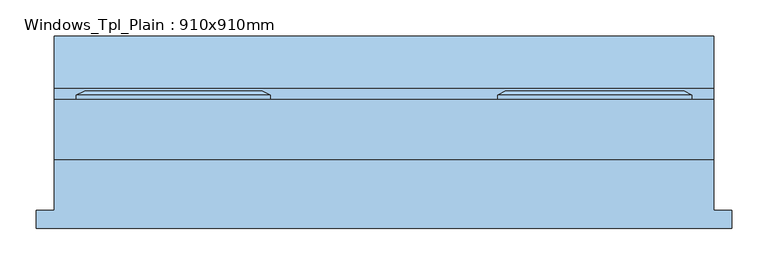
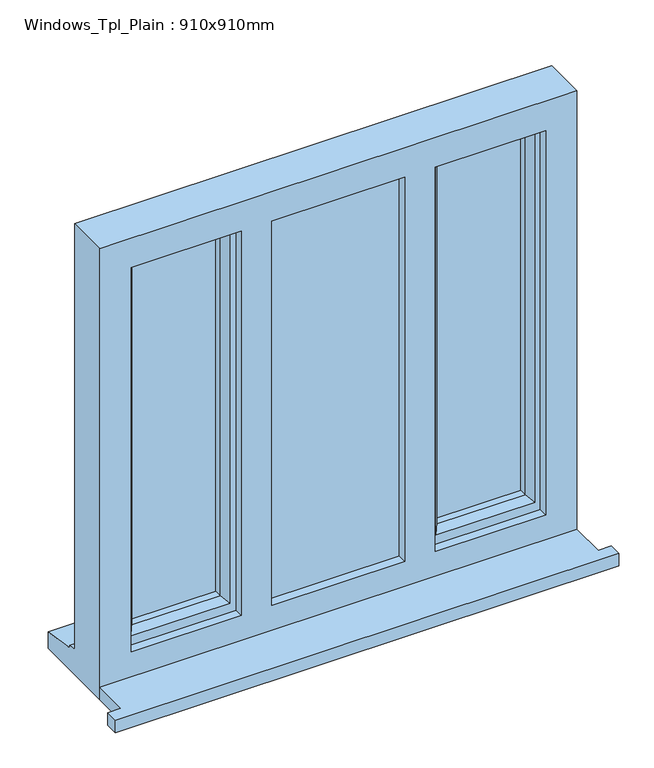
"""IFC4 building model written with IfcOpenShell, lengths in millimetres: window geometry, Windows_Tpl_Plain : 910x910mm."""

from ifc_helpers import new_model, si_unit, frame, origin, place, context, project, spatial, polyline, outline, extrude, faceted_brep, source, transform, mapped, element, save


def windows_tpl_plain_910x910mm_84e79c20(model_context):
    return source(origin(), model_context, "Body", "SolidModel", [
        extrude(outline(polyline([(-906.6666667, -118.1434322), (-906.6666667, -93.1434322), (-881.6666667, -93.1434322), (-881.6666667, -22.9434322), (28.3333333, -22.9434322), (28.3333333, -93.1434322), (53.3333333, -93.1434322), (53.3333333, -118.1434322), (-906.6666667, -118.1434322)])), frame((0.0, 0.0, 1200.0), z_axis=(0.0, 0.0, 1.0), x_axis=(1.0, 0.0, 0.0)), (0.0, 0.0, 1.0), 25.0),
        faceted_brep([(-270.0, 60.0565678, 2080.0), (-270.0, 65.8300705, 2080.0), (-270.0, 65.8300705, 1253.0), (-270.0, 60.0565678, 1253.0), (-260.0, -4.9434322, 2070.0), (-260.0, 60.0565678, 2070.0), (-260.0, 60.0565678, 1263.0), (-260.0, -4.9434322, 1263.0), (-220.0, 9.5494677, 2030.0), (-230.1480377, -4.9434322, 2040.1480377), (-230.1480377, -4.9434322, 1292.8519623), (-220.0, 9.5494677, 1303.0), (-220.0, 24.0565678, 2030.0), (-220.0, 24.0565678, 1303.0), (-230.0, 48.0565678, 2040.0), (-230.0, 24.0565678, 2040.0), (-230.0, 24.0565678, 1293.0), (-230.0, 48.0565678, 1293.0), (-220.0, 65.8300705, 2030.0), (-220.0, 48.0565678, 2030.0), (-220.0, 48.0565678, 1303.0), (-220.0, 65.8300705, 1303.0), (-237.4457548, 71.6035732, 2047.4457548), (-237.4457548, 71.6035732, 1285.5542452), (-259.2153903, 71.6035732, 2069.2153903), (-259.2153903, 71.6035732, 1263.7846097), (-1.6666667, 65.8300705, 1253.0), (-1.6666667, 60.0565678, 1253.0), (-11.6666667, 60.0565678, 1263.0), (-11.6666667, -4.9434322, 1263.0), (-41.5186289, -4.9434322, 1292.8519623), (-51.6666667, 9.5494677, 1303.0), (-51.6666667, 24.0565678, 1303.0), (-41.6666667, 24.0565678, 1293.0), (-41.6666667, 48.0565678, 1293.0), (-51.6666667, 48.0565678, 1303.0), (-51.6666667, 65.8300705, 1303.0), (-34.2209119, 71.6035732, 1285.5542452), (-12.4512764, 71.6035732, 1263.7846097), (-1.6666667, 65.8300705, 2080.0), (-1.6666667, 60.0565678, 2080.0), (-11.6666667, 60.0565678, 2070.0), (-11.6666667, -4.9434322, 2070.0), (-41.5186289, -4.9434322, 2040.1480377), (-51.6666667, 9.5494677, 2030.0), (-51.6666667, 24.0565678, 2030.0), (-41.6666667, 24.0565678, 2040.0), (-41.6666667, 48.0565678, 2040.0), (-51.6666667, 48.0565678, 2030.0), (-51.6666667, 65.8300705, 2030.0), (-34.2209119, 71.6035732, 2047.4457548), (-12.4512764, 71.6035732, 2069.2153903)], [[[0, 1, 2, 3]], [[4, 5, 6, 7]], [[8, 9, 10, 11]], [[12, 8, 11, 13]], [[14, 15, 16, 17]], [[18, 19, 20, 21]], [[22, 18, 21, 23]], [[1, 24, 25, 2]], [[3, 2, 26, 27]], [[7, 6, 28, 29]], [[11, 10, 30, 31]], [[13, 11, 31, 32]], [[17, 16, 33, 34]], [[21, 20, 35, 36]], [[23, 21, 36, 37]], [[2, 25, 38, 26]], [[27, 26, 39, 40]], [[29, 28, 41, 42]], [[31, 30, 43, 44]], [[32, 31, 44, 45]], [[34, 33, 46, 47]], [[36, 35, 48, 49]], [[37, 36, 49, 50]], [[26, 38, 51, 39]], [[40, 39, 1, 0]], [[3, 27, 40, 0], [5, 41, 28, 6]], [[42, 41, 5, 4]], [[7, 29, 42, 4], [9, 43, 30, 10]], [[44, 43, 9, 8]], [[45, 44, 8, 12]], [[15, 46, 33, 16], [13, 32, 45, 12]], [[47, 46, 15, 14]], [[17, 34, 47, 14], [19, 48, 35, 20]], [[49, 48, 19, 18]], [[50, 49, 18, 22]], [[24, 51, 38, 25], [23, 37, 50, 22]], [[39, 51, 24, 1]]]),
        faceted_brep([(-583.3333333, 60.0565678, 2080.0), (-583.3333333, 65.8300705, 2080.0), (-851.6666667, 65.8300705, 2080.0), (-851.6666667, 60.0565678, 2080.0), (-593.3333333, -4.9434322, 2070.0), (-593.3333333, 60.0565678, 2070.0), (-841.6666667, 60.0565678, 2070.0), (-841.6666667, -4.9434322, 2070.0), (-633.3333333, 9.5494677, 2030.0), (-623.1852956, -4.9434322, 2040.1480377), (-811.8147044, -4.9434322, 2040.1480377), (-801.6666667, 9.5494677, 2030.0), (-633.3333333, 24.0565678, 2030.0), (-801.6666667, 24.0565678, 2030.0), (-623.3333333, 48.0565678, 2040.0), (-623.3333333, 24.0565678, 2040.0), (-811.6666667, 24.0565678, 2040.0), (-811.6666667, 48.0565678, 2040.0), (-633.3333333, 65.8300705, 2030.0), (-633.3333333, 48.0565678, 2030.0), (-801.6666667, 48.0565678, 2030.0), (-801.6666667, 65.8300705, 2030.0), (-614.5187677, 71.6035732, 2048.8145656), (-820.4812323, 71.6035732, 2048.8145656), (-594.964114, 71.6035732, 2068.3692194), (-840.035886, 71.6035732, 2068.3692194), (-851.6666667, 65.8300705, 1253.0), (-851.6666667, 60.0565678, 1253.0), (-841.6666667, 60.0565678, 1263.0), (-841.6666667, -4.9434322, 1263.0), (-811.8147044, -4.9434322, 1292.8519623), (-801.6666667, 9.5494677, 1303.0), (-801.6666667, 24.0565678, 1303.0), (-811.6666667, 24.0565678, 1293.0), (-811.6666667, 48.0565678, 1293.0), (-801.6666667, 48.0565678, 1303.0), (-801.6666667, 65.8300705, 1303.0), (-820.4812323, 71.6035732, 1284.1854344), (-840.035886, 71.6035732, 1264.6307806), (-583.3333333, 65.8300705, 1253.0), (-583.3333333, 60.0565678, 1253.0), (-593.3333333, 60.0565678, 1263.0), (-593.3333333, -4.9434322, 1263.0), (-623.1852956, -4.9434322, 1292.8519623), (-633.3333333, 9.5494677, 1303.0), (-633.3333333, 24.0565678, 1303.0), (-623.3333333, 24.0565678, 1293.0), (-623.3333333, 48.0565678, 1293.0), (-633.3333333, 48.0565678, 1303.0), (-633.3333333, 65.8300705, 1303.0), (-614.5187677, 71.6035732, 1284.1854344), (-594.964114, 71.6035732, 1264.6307806)], [[[0, 1, 2, 3]], [[4, 5, 6, 7]], [[8, 9, 10, 11]], [[12, 8, 11, 13]], [[14, 15, 16, 17]], [[18, 19, 20, 21]], [[22, 18, 21, 23]], [[1, 24, 25, 2]], [[3, 2, 26, 27]], [[7, 6, 28, 29]], [[11, 10, 30, 31]], [[13, 11, 31, 32]], [[17, 16, 33, 34]], [[21, 20, 35, 36]], [[23, 21, 36, 37]], [[2, 25, 38, 26]], [[27, 26, 39, 40]], [[0, 3, 27, 40], [41, 28, 6, 5]], [[29, 28, 41, 42]], [[4, 7, 29, 42], [43, 30, 10, 9]], [[31, 30, 43, 44]], [[32, 31, 44, 45]], [[46, 33, 16, 15], [12, 13, 32, 45]], [[34, 33, 46, 47]], [[14, 17, 34, 47], [48, 35, 20, 19]], [[36, 35, 48, 49]], [[37, 36, 49, 50]], [[51, 38, 25, 24], [22, 23, 37, 50]], [[26, 38, 51, 39]], [[40, 39, 1, 0]], [[42, 41, 5, 4]], [[44, 43, 9, 8]], [[45, 44, 8, 12]], [[47, 46, 15, 14]], [[49, 48, 19, 18]], [[50, 49, 18, 22]], [[39, 51, 24, 1]]]),
        faceted_brep([(28.3333333, -22.9434322, 2110.0), (-881.6666667, -22.9434322, 2110.0), (-881.6666667, -22.9434322, 1200.0), (28.3333333, -22.9434322, 1200.0), (-31.6666667, -22.9434322, 2050.0), (-31.6666667, -22.9434322, 1275.0), (-242.0, -22.9434322, 1275.0), (-242.0, -22.9434322, 2050.0), (-300.0, -22.9434322, 2050.0), (-300.0, -22.9434322, 1275.0), (-553.3333333, -22.9434322, 1275.0), (-553.3333333, -22.9434322, 2050.0), (-611.3333333, -22.9434322, 2050.0), (-611.3333333, -22.9434322, 1275.0), (-821.6666667, -22.9434322, 1275.0), (-821.6666667, -22.9434322, 2050.0), (-881.6666667, 60.0565678, 2110.0), (-881.6666667, 60.0565678, 1251.0), (-881.6666667, 75.0565678, 1249.68767), (-881.6666667, 75.0565678, 1244.7449676), (-881.6666667, 147.5565678, 1233.8088847), (-881.6666667, 147.5565678, 1200.0), (28.3333333, 60.0565678, 2110.0), (28.3333333, 60.0565678, 1251.0), (-841.6666667, 60.0565678, 2070.0), (-841.6666667, 60.0565678, 1263.0), (-593.3333333, 60.0565678, 1263.0), (-593.3333333, 60.0565678, 2070.0), (-553.3333333, 60.0565678, 2070.0), (-553.3333333, 60.0565678, 1263.0), (-300.0, 60.0565678, 1263.0), (-300.0, 60.0565678, 2070.0), (-260.0, 60.0565678, 2070.0), (-260.0, 60.0565678, 1263.0), (-11.6666667, 60.0565678, 1263.0), (-11.6666667, 60.0565678, 2070.0), (-841.6666667, -4.9434322, 2070.0), (-841.6666667, -4.9434322, 1263.0), (-563.3333333, -4.9434322, 2070.0), (-290.0, -4.9434322, 2070.0), (-290.0, -4.9434322, 1263.0), (-563.3333333, -4.9434322, 1263.0), (-300.0, -4.9434322, 2050.0), (-553.3333333, -4.9434322, 2050.0), (-553.3333333, -4.9434322, 1275.0), (-300.0, -4.9434322, 1275.0), (-260.0, -4.9434322, 2070.0), (-11.6666667, -4.9434322, 2070.0), (-11.6666667, -4.9434322, 1263.0), (-260.0, -4.9434322, 1263.0), (-31.6666667, -4.9434322, 2050.0), (-242.0, -4.9434322, 2050.0), (-242.0, -4.9434322, 1275.0), (-31.6666667, -4.9434322, 1275.0), (-593.3333333, -4.9434322, 2070.0), (-593.3333333, -4.9434322, 1263.0), (-611.3333333, -4.9434322, 2050.0), (-821.6666667, -4.9434322, 2050.0), (-821.6666667, -4.9434322, 1275.0), (-611.3333333, -4.9434322, 1275.0), (-553.3333333, 19.0565678, 2070.0), (-300.0, 19.0565678, 2070.0), (-290.0, 19.0565678, 2070.0), (-563.3333333, 19.0565678, 2070.0), (28.3333333, 147.5565678, 1200.0), (28.3333333, 147.5565678, 1233.8088847), (28.3333333, 75.0565678, 1244.7449676), (28.3333333, 75.0565678, 1249.68767), (-553.3333333, 19.0565678, 1263.0), (-563.3333333, 19.0565678, 1263.0), (-290.0, 19.0565678, 1263.0), (-300.0, 19.0565678, 1263.0)], [[[0, 1, 2, 3], [4, 5, 6, 7], [8, 9, 10, 11], [12, 13, 14, 15]], [[2, 1, 16, 17, 18, 19, 20, 21]], [[17, 16, 22, 23], [24, 25, 26, 27], [28, 29, 30, 31], [32, 33, 34, 35]], [[25, 24, 36, 37]], [[38, 39, 40, 41], [42, 43, 44, 45]], [[46, 47, 48, 49], [50, 51, 52, 53]], [[36, 54, 55, 37], [56, 57, 58, 59]], [[57, 15, 14, 58]], [[1, 0, 22, 16]], [[36, 24, 27, 54]], [[35, 47, 46, 32]], [[60, 28, 31, 61, 62, 39, 38, 63]], [[15, 57, 56, 12]], [[50, 4, 7, 51]], [[11, 43, 42, 8]], [[23, 22, 0, 3, 64, 65, 66, 67]], [[35, 34, 48, 47]], [[4, 50, 53, 5]], [[43, 11, 10, 44]], [[12, 56, 59, 13]], [[27, 26, 55, 54]], [[29, 28, 60, 68]], [[68, 60, 63, 69]], [[69, 63, 38, 41]], [[62, 70, 40, 39]], [[70, 62, 61, 71]], [[71, 61, 31, 30]], [[33, 32, 46, 49]], [[51, 7, 6, 52]], [[8, 42, 45, 9]], [[64, 3, 2, 21]], [[65, 64, 21, 20]], [[66, 65, 20, 19]], [[67, 66, 19, 18]], [[23, 67, 18, 17]], [[26, 25, 37, 55]], [[34, 33, 49, 48]], [[41, 40, 70, 71, 30, 29, 68, 69]], [[6, 5, 53, 52]], [[45, 44, 10, 9]], [[59, 58, 14, 13]]]),
        extrude(outline(polyline([(-623.3333333, 24.0565678), (-811.6666667, 24.0565678), (-811.6666667, 48.0565678), (-623.3333333, 48.0565678), (-623.3333333, 24.0565678)])), frame((0.0, 0.0, 1293.0), z_axis=(0.0, 0.0, 1.0), x_axis=(1.0, 0.0, 0.0)), (0.0, 0.0, 1.0), 747.0),
        extrude(outline(polyline([(-563.3333333, 19.0565678), (-290.0, 19.0565678), (-290.0, -4.9434322), (-563.3333333, -4.9434322), (-563.3333333, 19.0565678)])), frame((0.0, 0.0, 1263.0), z_axis=(0.0, 0.0, 1.0), x_axis=(1.0, 0.0, 0.0)), (0.0, 0.0, 1.0), 807.0),
        extrude(outline(polyline([(-41.6666667, 24.0565678), (-230.0, 24.0565678), (-230.0, 48.0565678), (-41.6666667, 48.0565678), (-41.6666667, 24.0565678)])), frame((0.0, 0.0, 1293.0), z_axis=(0.0, 0.0, 1.0), x_axis=(1.0, 0.0, 0.0)), (0.0, 0.0, 1.0), 747.0),
    ])


if __name__ == "__main__":
    model = new_model("IFC4")
    model_context = context("Model", 3, world=origin())
    ifc_project = project(units=[si_unit("LENGTHUNIT", "METRE", prefix="MILLI")], contexts=[model_context])
    site = spatial("IfcSite", under=ifc_project)
    building = spatial("IfcBuilding", under=site)
    placement = place(None, origin())
    windows_tpl_plain_910x910mm_shape = windows_tpl_plain_910x910mm_84e79c20(model_context)
    element("IfcWindow", 1, ObjectType="Windows_Tpl_Plain : 910x910mm", at=placement, inside=building, context=model_context, shape_type="MappedRepresentation", body=[
        mapped(windows_tpl_plain_910x910mm_shape, transform((0.0, 0.0, 0.0), x_axis=(1.0, 0.0, 0.0), y_axis=(0.0, 1.0, 0.0), z_axis=(0.0, 0.0, 1.0))),
    ])
    save(model, "model.ifc")

# Revit data of these elements
# Type "Windows_Tpl_Plain : 910x910mm"
#   Type Mark = "24"
#   Operation = "TriplePanelVertical"
#   Construction Type Id = "GSP4R"
#   Manufacturer = "Revit"
#   Keynote = "L10"
#   Analytic Construction = "1/8 in Pilkington single glazing"
#   Wrap Layers (Ext) from Ext = 0' - 4.03543"
#   Wrap Layers (Int) from Ext = 0' - 6.98819"
#   Window Board Projection = 0' - 0.98425"
#   Window Board Extension = 0' - 0.98425"
#   Visual Light Transmittance = 0.9
#   Solar Heat Gain Coefficient = 0.78
#   Rough Width = 2' - 11.82677"
#   Rough Height = 2' - 11.82677"
#   Height = 2' - 11.82677"
#   Width = 2' - 11.82677"
#   Heat Transfer Coefficient (U) = 0.6496 BTU/(h·ft²·°F)
#   Glazing Thickness = 0' - 0.94488"
#   FrameOffset - External = 0' - 1.9685"
#   Frame Depth = 0' - 2.55906"
#   Default Head Height = 6' - 11.07087"
#   Cill Depth = 0' - 3.44488"
#   Cavity Closer Width = 0' - 1.9685"
#   Cavity Closer Offset from Ext = 0' - 4.03543"
#   Cavity Closer Depth = 0' - 3.34646"
#   Vis - Cavity Closers = yes
#   Define Thermal Properties by = 1
#   Material Trim = Window Frame
#   Material Glass = Glass
#   Material Frame = Window Frame
#   Wall Closure = (empty or 0)
# Element 1 (IfcWindow, "Windows_Tpl_Plain : 910x910mm")
#   Materials on its faces: "Window Frame", "Glass"
# Materials
#   "Window Frame": colour RGB 249 249 249, transparency 0
#   "Glass": class "Glass", colour RGB 0 128 192, transparency 0.75, Description = "Soda Lime Glass", Cost = 0
